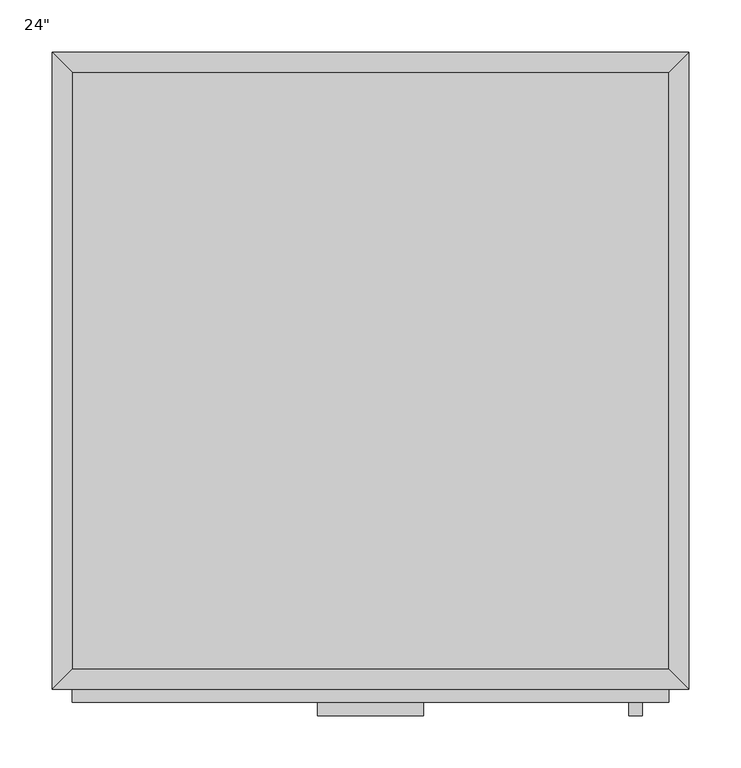
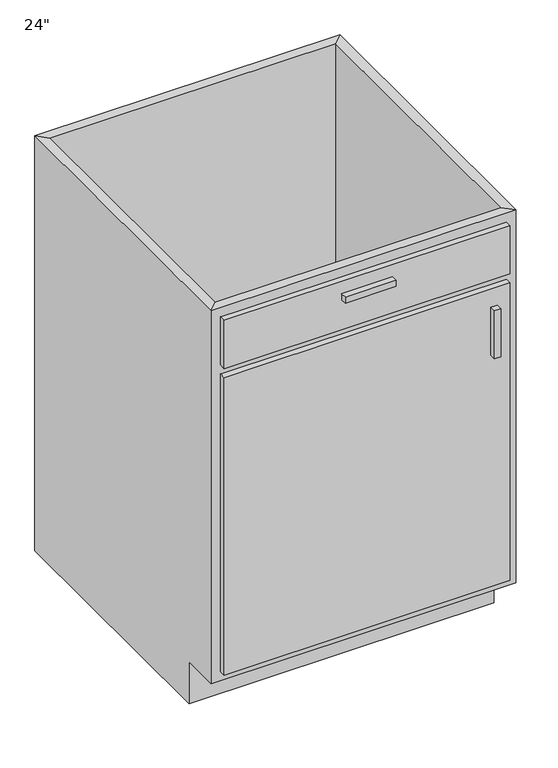
"""IFC4 building model written with IfcOpenShell, lengths in millimetres: furniture geometry."""

from ifc_helpers import new_model, si_unit, frame, origin, place, context, project, spatial, polyline, outline, extrude, faceted_brep, source, transform, mapped, element, save


def furniture_6a014568(model_context):
    return source(origin(), model_context, "Body", "SolidModel", [
        faceted_brep([(304.4877049, -590.55, 876.3), (304.4877049, -590.55, 88.9), (-267.0122951, -590.55, 88.9), (-267.0122951, -590.55, 876.3), (-286.0622951, -609.6, 876.3), (323.5377049, -609.6, 876.3), (-286.0622951, -609.6, 88.9), (323.5377049, -609.6, 88.9), (-267.0122951, -533.4, 88.9), (-267.0122951, -19.05, 88.9), (-267.0122951, -19.05, 876.3), (-286.0622951, 0.0, 876.3), (-286.0622951, 0.0, 0.0), (-286.0622951, -533.4, 0.0), (-286.0622951, -533.4, 88.9), (304.4877049, -19.05, 88.9), (304.4877049, -19.05, 876.3), (323.5377049, 0.0, 876.3), (323.5377049, 0.0, 0.0), (304.4877049, -533.4, 88.9), (323.5377049, -533.4, 88.9), (323.5377049, -533.4, 0.0)], [[[0, 1, 2, 3]], [[0, 3, 4, 5]], [[5, 4, 6, 7]], [[2, 1, 7, 6]], [[3, 2, 8, 9, 10]], [[4, 3, 10, 11]], [[6, 4, 11, 12, 13, 14]], [[2, 6, 14, 8]], [[10, 9, 15, 16]], [[11, 10, 16, 17]], [[12, 11, 17, 18]], [[1, 0, 16, 15, 19]], [[0, 5, 17, 16]], [[5, 7, 20, 21, 18, 17]], [[7, 1, 19, 20]], [[8, 19, 15, 9]], [[18, 21, 13, 12]], [[13, 21, 20, 19, 8, 14]]]),
        extrude(outline(polyline([(279.0877049, -635.0), (266.3877049, -635.0), (266.3877049, -622.3), (279.0877049, -622.3), (279.0877049, -635.0)])), frame((0.0, 0.0, 596.9), z_axis=(0.0, 0.0, 1.0), x_axis=(1.0, 0.0, 0.0)), (0.0, 0.0, 1.0), 101.6),
        extrude(outline(polyline([(69.5377049, -635.0), (-32.0622951, -635.0), (-32.0622951, -622.3), (69.5377049, -622.3), (69.5377049, -635.0)])), frame((0.0, 0.0, 819.15), z_axis=(0.0, 0.0, 1.0), x_axis=(1.0, 0.0, 0.0)), (0.0, 0.0, 1.0), 12.7),
        extrude(outline(polyline([(304.4877049, -622.3), (-267.0122951, -622.3), (-267.0122951, -609.6), (304.4877049, -609.6), (304.4877049, -622.3)])), frame((0.0, 0.0, 107.95), z_axis=(0.0, 0.0, 1.0), x_axis=(1.0, 0.0, 0.0)), (0.0, 0.0, 1.0), 628.65),
        extrude(outline(polyline([(304.4877049, -622.3), (-267.0122951, -622.3), (-267.0122951, -609.6), (304.4877049, -609.6), (304.4877049, -622.3)])), frame((0.0, 0.0, 755.65), z_axis=(0.0, 0.0, 1.0), x_axis=(1.0, 0.0, 0.0)), (0.0, 0.0, 1.0), 101.6),
        extrude(outline(polyline([(304.4877049, -19.05), (304.4877049, -590.55), (-267.0122951, -590.55), (-267.0122951, -19.05), (304.4877049, -19.05)])), frame((0.0, 0.0, 88.9), z_axis=(0.0, 0.0, 1.0), x_axis=(1.0, 0.0, 0.0)), (0.0, 0.0, 1.0), 19.05),
    ])


if __name__ == "__main__":
    model = new_model("IFC4")
    model_context = context("Model", 3, world=origin())
    ifc_project = project(units=[si_unit("LENGTHUNIT", "METRE", prefix="MILLI")], contexts=[model_context])
    site = spatial("IfcSite", under=ifc_project)
    building = spatial("IfcBuilding", under=site)
    placement = place(None, origin())
    furniture_shape = furniture_6a014568(model_context)
    element("IfcFurniture", 1, ObjectType="24\"", at=placement, inside=building, context=model_context, shape_type="MappedRepresentation", body=[
        mapped(furniture_shape, transform((0.0, 0.0, 0.0), x_axis=(1.0, 0.0, 0.0), y_axis=(0.0, 1.0, 0.0), z_axis=(0.0, 0.0, 1.0))),
    ])
    save(model, "model.ifc")

# Revit data of these elements
# Type "24\""
#   Assembly Code = "C1030410"
#   Depth = 2' - 0"
#   Height = 2' - 10 1/2"
#   Toe Depth = 0' - 3"
#   Toe Height = 0' - 3 1/2"
#   Width = 2' - 0"
#   Cabinet Material = none
#   Drawer Material = none
#   Handle Material = Cabinets - Handles
#   Default Elevation = 0
# Element 1 (IfcFurniture, "24\"")
#   Materials on its faces: "Cabinets", "Cabinets - Handles"
# Materials
#   "Cabinets - Handles": class "Metal", colour RGB 57 57 57, transparency 0
#   "Cabinets": colour RGB 249 249 249, transparency 0
